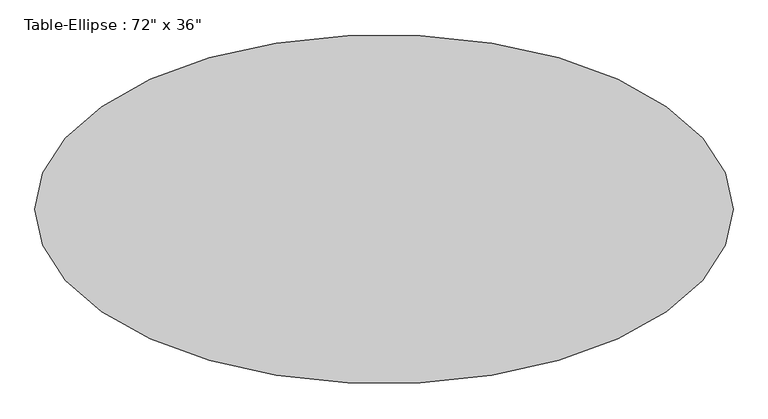
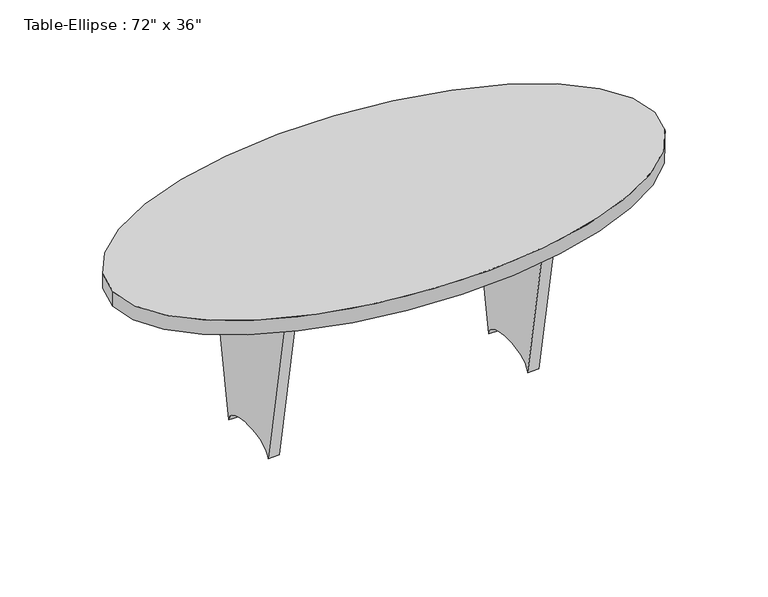
"""IFC4 building model written with IfcOpenShell, lengths in millimetres: furniture geometry."""

from ifc_helpers import new_model, si_unit, point, frame, origin, place, context, project, spatial, ellipse_curve, trimmed, source, transform, mapped, element, save
from ifc_brep_helpers import plane_surface, extruded_surface, advanced_brep


def furniture_0791916c(model_context):
    return source(origin(), model_context, "Body", "AdvancedBrep", [
        advanced_brep(
        [(-419.1, 19.05, 635.0), (419.1, 19.05, 635.0), (419.1, 19.05, 423.3333333), (-419.1, 19.05, 423.3333333), (-419.1, -19.05, 635.0), (-419.1, -19.05, 423.3333333), (419.1, -19.05, 423.3333333), (419.1, -19.05, 635.0)],
        [
            (0, 1),
            (1, 2),
            (2, 3, ellipse_curve(frame((0.0, 19.05, 423.3333333), z_axis=(0.0, -1.0, 0.0), x_axis=(1.0, 0.0, 0.0)), 419.1, 101.6)),
            (3, 0),
            (4, 5),
            (5, 6, ellipse_curve(frame((0.0, -19.05, 423.3333333), z_axis=(0.0, 1.0, 0.0), x_axis=(1.0, 0.0, 0.0)), 419.1, 101.6)),
            (6, 7),
            (7, 4),
            (0, 4),
            (7, 1),
            (6, 2),
            (5, 3),
        ],
        [
            plane_surface(frame((-419.1, 19.05, 635.0), z_axis=(0.0, 1.0, 0.0), x_axis=(1.0, 0.0, 0.0))),
            plane_surface(frame((-419.1, -19.05, 635.0), z_axis=(0.0, -1.0, 0.0), x_axis=(-1.0, 0.0, 0.0))),
            plane_surface(frame((-419.1, 19.05, 635.0), z_axis=(0.0, 0.0, 1.0), x_axis=(0.0, -1.0, 0.0))),
            plane_surface(frame((419.1, 19.05, 635.0), z_axis=(1.0, 0.0, 0.0), x_axis=(0.0, -1.0, 0.0))),
            extruded_surface(trimmed(ellipse_curve(frame((0.0, -57.15, 423.3333333), z_axis=(0.0, -1.0, 0.0), x_axis=(1.0, 0.0, 0.0)), 419.1, 101.6), [point((419.1, -57.15, 423.3333333))], [point((-419.1, -57.15, 423.3333333))], True, "CARTESIAN"), (0.0, 38.099999999999994, 0.0), 38.099999999999994),
            plane_surface(frame((-419.1, 19.05, 423.3333333), z_axis=(-1.0, 0.0, 0.0), x_axis=(0.0, -1.0, 0.0))),
        ],
        [
            (0, [[1, 2, 3, 4]]),
            (1, [[5, 6, 7, 8]]),
            (2, [[-1, 9, -8, 10]]),
            (3, [[-2, -10, -7, 11]]),
            (4, [[-3, -11, -6, 12]]),
            (5, [[-4, -12, -5, -9]]),
        ],
    ),
        advanced_brep(
        [(457.2, 228.6, 635.0), (457.2, -228.6, 635.0), (457.2, -114.3, 0.0), (457.2, 114.3, 0.0), (419.1, 228.6, 635.0), (419.1, 114.3, 0.0), (419.1, -114.3, 0.0), (419.1, -228.6, 635.0)],
        [
            (0, 1),
            (1, 2),
            (2, 3, ellipse_curve(frame((457.2, 0.0, 0.0), z_axis=(-1.0, 0.0, 0.0), x_axis=(0.0, 1.0, 0.0)), 114.3, 50.8)),
            (3, 0),
            (4, 5),
            (5, 6, ellipse_curve(frame((419.1, 0.0, 0.0), z_axis=(1.0, 0.0, 0.0), x_axis=(0.0, 1.0, 0.0)), 114.3, 50.8)),
            (6, 7),
            (7, 4),
            (0, 4),
            (7, 1),
            (6, 2),
            (5, 3),
        ],
        [
            plane_surface(frame((457.2, -228.6, 635.0), z_axis=(1.0, 0.0, 0.0), x_axis=(0.0, -1.0, 0.0))),
            plane_surface(frame((419.1, -228.6, 635.0), z_axis=(-1.0, 0.0, 0.0), x_axis=(0.0, 1.0, 0.0))),
            plane_surface(frame((457.2, 228.6, 635.0), z_axis=(0.0, 0.0, 1.0), x_axis=(-1.0, 0.0, 0.0))),
            plane_surface(frame((457.2, -228.6, 635.0), z_axis=(0.0, -0.9841833239736941, -0.17715299831527212), x_axis=(-1.0, 0.0, 0.0))),
            extruded_surface(trimmed(ellipse_curve(frame((381.0, 0.0, 0.0), z_axis=(-1.0, 0.0, 0.0), x_axis=(0.0, 1.0, 0.0)), 114.3, 50.8), [point((381.0, -114.3, 0.0))], [point((381.0, 114.3, 0.0))], True, "CARTESIAN"), (38.10000000000002, 0.0, 0.0), 38.10000000000002),
            plane_surface(frame((457.2, 114.3, 0.0), z_axis=(0.0, 0.984183323973697, -0.17715299831525538), x_axis=(-1.0, 0.0, 0.0))),
        ],
        [
            (0, [[1, 2, 3, 4]]),
            (1, [[5, 6, 7, 8]]),
            (2, [[-1, 9, -8, 10]]),
            (3, [[-2, -10, -7, 11]]),
            (4, [[-3, -11, -6, 12]]),
            (5, [[-4, -12, -5, -9]]),
        ],
    ),
        advanced_brep(
        [(-419.1, 228.6, 635.0), (-419.1, -228.6, 635.0), (-419.1, -114.3, 0.0), (-419.1, 114.3, 0.0), (-457.2, 228.6, 635.0), (-457.2, 114.3, 0.0), (-457.2, -114.3, 0.0), (-457.2, -228.6, 635.0)],
        [
            (0, 1),
            (1, 2),
            (2, 3, ellipse_curve(frame((-419.1, 0.0, 0.0), z_axis=(-1.0, 0.0, 0.0), x_axis=(0.0, 1.0, 0.0)), 114.3, 50.8)),
            (3, 0),
            (4, 5),
            (5, 6, ellipse_curve(frame((-457.2, 0.0, 0.0), z_axis=(1.0, 0.0, 0.0), x_axis=(0.0, 1.0, 0.0)), 114.3, 50.8)),
            (6, 7),
            (7, 4),
            (0, 4),
            (7, 1),
            (6, 2),
            (5, 3),
        ],
        [
            plane_surface(frame((-419.1, -228.6, 635.0), z_axis=(1.0, 0.0, 0.0), x_axis=(0.0, -1.0, 0.0))),
            plane_surface(frame((-457.2, -228.6, 635.0), z_axis=(-1.0, 0.0, 0.0), x_axis=(0.0, 1.0, 0.0))),
            plane_surface(frame((-419.1, 228.6, 635.0), z_axis=(0.0, 0.0, 1.0), x_axis=(-1.0, 0.0, 0.0))),
            plane_surface(frame((-419.1, -228.6, 635.0), z_axis=(0.0, -0.9841833239736942, -0.17715299831527118), x_axis=(-1.0, 0.0, 0.0))),
            extruded_surface(trimmed(ellipse_curve(frame((-495.3, 0.0, 0.0), z_axis=(-1.0, 0.0, 0.0), x_axis=(0.0, 1.0, 0.0)), 114.3, 50.8), [point((-495.3, -114.3, 0.0))], [point((-495.3, 114.3, 0.0))], True, "CARTESIAN"), (38.10000000000002, 0.0, 0.0), 38.10000000000002),
            plane_surface(frame((-419.1, 114.3, 0.0), z_axis=(0.0, 0.9841833239736961, -0.1771529983152611), x_axis=(-1.0, 0.0, 0.0))),
        ],
        [
            (0, [[1, 2, 3, 4]]),
            (1, [[5, 6, 7, 8]]),
            (2, [[-1, 9, -8, 10]]),
            (3, [[-2, -10, -7, 11]]),
            (4, [[-3, -11, -6, 12]]),
            (5, [[-4, -12, -5, -9]]),
        ],
    ),
        advanced_brep(
        [(-914.4, 0.0, 685.8), (914.4, 0.0, 685.8), (-914.4, 0.0, 635.0), (914.4, 0.0, 635.0)],
        [
            (0, 1, ellipse_curve(frame((0.0, 0.0, 685.8), z_axis=(0.0, 0.0, 1.0), x_axis=(1.0, 0.0, 0.0)), 914.4, 457.2)),
            (1, 0, ellipse_curve(frame((0.0, 0.0, 685.8), z_axis=(0.0, 0.0, 1.0), x_axis=(1.0, 0.0, 0.0)), 914.4, 457.2)),
            (2, 3, ellipse_curve(frame((0.0, 0.0, 635.0), z_axis=(0.0, 0.0, -1.0), x_axis=(1.0, 0.0, 0.0)), 914.4, 457.2)),
            (3, 2, ellipse_curve(frame((0.0, 0.0, 635.0), z_axis=(0.0, 0.0, -1.0), x_axis=(1.0, 0.0, 0.0)), 914.4, 457.2)),
            (0, 2),
            (3, 1),
        ],
        [
            plane_surface(frame((914.4, 0.0, 685.8), z_axis=(0.0, 0.0, 1.0), x_axis=(0.0, 1.0, 0.0))),
            plane_surface(frame((914.4, 0.0, 635.0), z_axis=(0.0, 0.0, -1.0), x_axis=(0.0, -1.0, 0.0))),
            extruded_surface(trimmed(ellipse_curve(frame((0.0, 0.0, 584.2), z_axis=(0.0, 0.0, 1.0), x_axis=(1.0, 0.0, 0.0)), 914.4, 457.2), [point((-914.4, 0.0, 584.2))], [point((914.4, 0.0, 584.2))], True, "CARTESIAN"), (0.0, 0.0, 50.799999999999955), 50.799999999999955),
            extruded_surface(trimmed(ellipse_curve(frame((0.0, 0.0, 584.2), z_axis=(0.0, 0.0, 1.0), x_axis=(1.0, 0.0, 0.0)), 914.4, 457.2), [point((914.4, 0.0, 584.2))], [point((-914.4, 0.0, 584.2))], True, "CARTESIAN"), (0.0, 0.0, 50.799999999999955), 50.799999999999955),
        ],
        [
            (0, [[1, 2]]),
            (1, [[3, 4]]),
            (2, [[-1, 5, -4, 6]]),
            (3, [[-2, -6, -3, -5]]),
        ],
    ),
    ])


if __name__ == "__main__":
    model = new_model("IFC4")
    model_context = context("Model", 3, world=origin())
    ifc_project = project(units=[si_unit("LENGTHUNIT", "METRE", prefix="MILLI")], contexts=[model_context])
    site = spatial("IfcSite", under=ifc_project)
    building = spatial("IfcBuilding", under=site)
    placement = place(None, origin())
    furniture_shape = furniture_0791916c(model_context)
    element("IfcFurniture", 1, ObjectType="Table-Ellipse : 72\" x 36\"", at=placement, inside=building, context=model_context, shape_type="MappedRepresentation", body=[
        mapped(furniture_shape, transform((0.0, 0.0, 0.0), x_axis=(1.0, 0.0, 0.0), y_axis=(0.0, 1.0, 0.0), z_axis=(0.0, 0.0, 1.0))),
    ])
    save(model, "model.ifc")

# Revit data of these elements
# Type "Table-Ellipse : 72\" x 36\""
#   Assembly Code = "E2020200"
#   Half Width = 1' - 6"
#   Half Length = 3' - 0"
#   Height = 2' - 3"
#   Length = 6' - 0"
#   Width = 3' - 0"
#   Base Material = Birch
#   Top Material = Plywood, Sheathing
#   Default Elevation = 0
# Element 1 (IfcFurniture, "Table-Ellipse : 72\" x 36\"")
#   Materials on its faces: "Birch", "Plywood, Sheathing"
# Materials
#   "Birch": class "Wood", colour RGB 210 159 95, transparency 0, Description = "Betula Alleghaniensis", Cost = 0
#   "Plywood, Sheathing": class "Wood", colour RGB 212 179 113, transparency 0, Description = "Plywood, sheathing grade", Cost = 0
